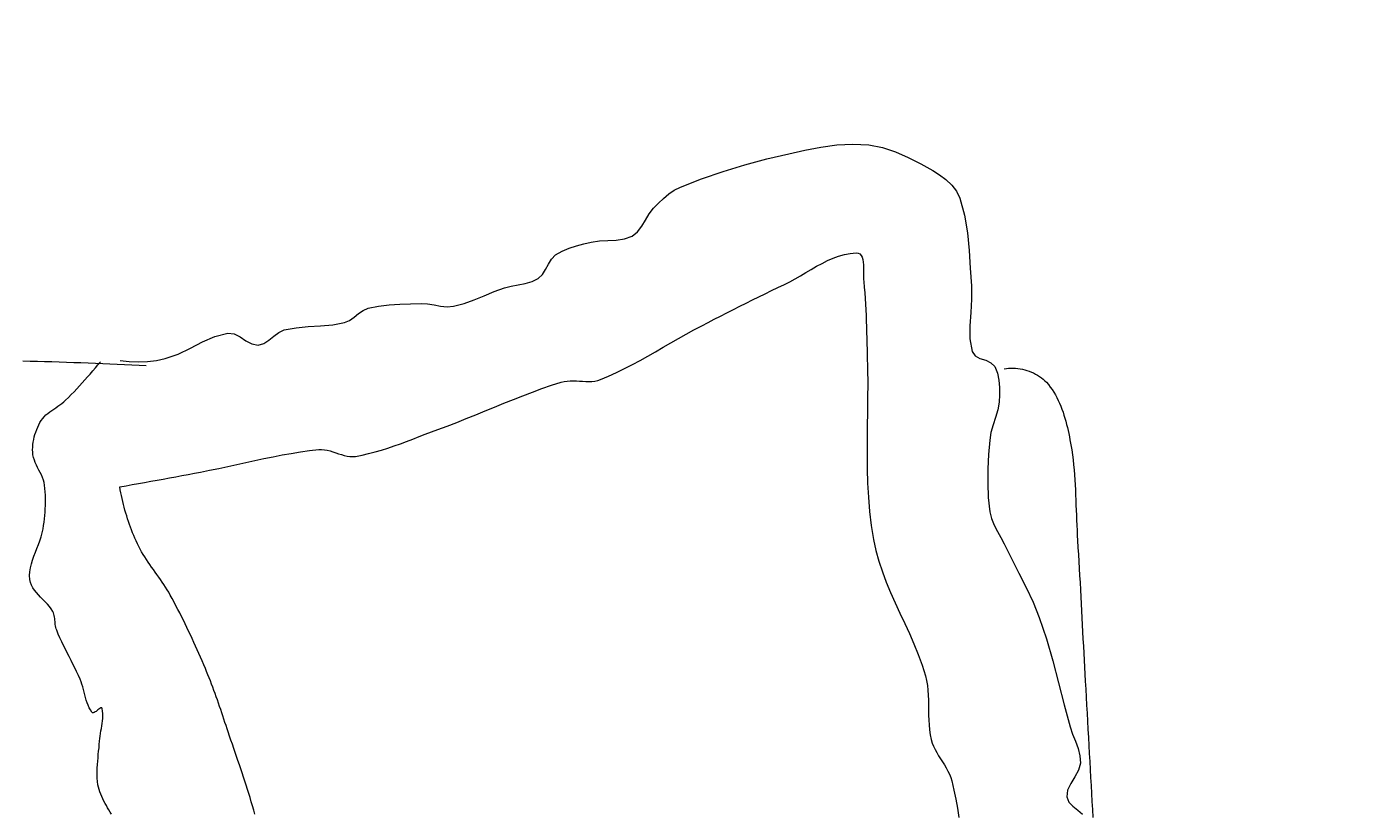
# Model space of a CAD drawing. Units: inches. Extents: x 1441 to 2460, y 1648 to 2683.
# Tile 8 of 35: x 1852 to 1880, y 1917 to 1933. Entities that reach past the tile are written whole.
import ezdxf

# ---------------------------------------------------------------- set-up
doc = ezdxf.new("R2010")
doc.units = ezdxf.units.IN
doc.layers.add('A-ANNO-DIMS', color=2, linetype='Continuous', lineweight=18)
doc.layers.add('A-FURN', color=8, linetype='Continuous', lineweight=15)
doc.styles.get("Standard").update_dxf_attribs({"font": 'arial.ttf'})
doc.dimstyles.get("Standard").update_dxf_attribs({"dimtxt": 0.18, "dimasz": 0.18, "dimexe": 0.18, "dimexo": 0.0625, "dimgap": 0.09, "dimtad": 0, "dimtih": 1, "dimtoh": 1, "dimdec": 4, "dimzin": 0, "dimdsep": 46, "dimtxsty": 'Standard', "dimcen": 0.09, "dimadec": 0, "dimazin": 0, "dimtfac": 1, "dimtdec": 4, "dimtofl": 0, "dimtmove": 0, "dimatfit": 3, "dimfxl": 1, "dimtolj": 1, "dimtzin": 0, "dimarcsym": 0})

# ---------------------------------------------------------------- blocks, each defined once
blk = doc.blocks.new('BED-DOUBLE-PLAN')
for p, q in [((13.358, 86.279), (13.525, 86.288)), ((13.525, 86.288), (13.692, 86.298)), ((13.692, 86.298), (13.859, 86.307)), ((13.859, 86.307), (14.025, 86.316)), ((14.025, 86.316), (14.192, 86.326)), ((14.192, 86.326), (14.359, 86.335)), ((14.359, 86.335), (14.526, 86.344)), ((14.526, 86.344), (14.693, 86.354)), ((14.693, 86.354), (14.859, 86.363)), ((14.859, 86.363), (15.026, 86.373)), ((15.026, 86.373), (15.193, 86.382)), ((15.193, 86.382), (15.36, 86.392)), ((8.125, 86), (8.23, 86.008)), ((8.23, 86.008), (8.334, 86.016)), ((8.334, 86.016), (8.439, 86.022)), ((8.439, 86.022), (8.544, 86.028)), ((8.544, 86.028), (8.649, 86.032)), ((8.649, 86.032), (8.755, 86.037)), ((8.755, 86.037), (8.86, 86.04)), ((8.86, 86.04), (8.965, 86.044)), ((8.965, 86.044), (9.07, 86.048)), ((9.07, 86.048), (9.175, 86.052)), ((9.175, 86.052), (9.281, 86.056)), ((9.281, 86.056), (9.386, 86.061)), ((9.386, 86.061), (9.491, 86.066)), ((9.491, 86.066), (9.595, 86.072)), ((9.595, 86.072), (9.742, 86.081)), ((9.742, 86.081), (9.888, 86.09)), ((9.888, 86.09), (10.035, 86.099)), ((10.035, 86.099), (10.181, 86.107)), ((10.181, 86.107), (10.327, 86.116)), ((10.327, 86.116), (10.474, 86.124)), ((10.474, 86.124), (10.62, 86.132)), ((10.62, 86.132), (10.767, 86.14)), ((10.767, 86.14), (10.913, 86.147)), ((10.913, 86.147), (11.059, 86.155)), ((11.059, 86.155), (11.206, 86.163)), ((11.206, 86.163), (11.352, 86.17)), ((11.352, 86.17), (11.499, 86.178)), ((11.499, 86.178), (11.645, 86.185)), ((11.645, 86.185), (11.792, 86.193)), ((11.792, 86.193), (11.938, 86.201)), ((11.938, 86.201), (12.085, 86.209)), ((12.085, 86.209), (12.231, 86.216)), ((12.231, 86.216), (12.377, 86.224)), ((12.377, 86.224), (12.524, 86.232)), ((12.524, 86.232), (12.691, 86.242)), ((12.691, 86.242), (12.858, 86.251)), ((12.858, 86.251), (13.024, 86.26)), ((13.024, 86.26), (13.191, 86.27)), ((13.191, 86.27), (13.358, 86.279)), ((13.624, 85.969), (13.774, 86.028)), ((13.774, 86.028), (13.925, 86.082)), ((13.925, 86.082), (14.077, 86.121)), ((14.077, 86.121), (14.232, 86.132)), ((14.232, 86.132), (14.378, 86.095)), ((14.378, 86.095), (14.515, 86.019)), ((14.515, 86.019), (14.65, 85.933)), ((15.126, 85.971), (15.205, 86.075)), ((15.205, 86.075), (15.287, 86.175)), ((6.802, 85.724), (6.864, 85.748)), ((6.864, 85.748), (6.926, 85.77)), ((6.926, 85.77), (6.989, 85.79)), ((6.989, 85.79), (7.053, 85.809)), ((7.053, 85.809), (7.117, 85.827)), ((7.117, 85.827), (7.181, 85.844)), ((7.181, 85.844), (7.246, 85.86)), ((7.246, 85.86), (7.31, 85.874)), ((7.31, 85.874), (7.374, 85.888)), ((7.374, 85.888), (7.438, 85.902)), ((7.438, 85.902), (7.502, 85.915)), ((7.502, 85.915), (7.605, 85.934)), ((7.605, 85.934), (7.709, 85.951)), ((7.709, 85.951), (7.812, 85.966)), ((7.812, 85.966), (7.916, 85.979)), ((7.916, 85.979), (8.021, 85.99)), ((8.021, 85.99), (8.125, 86)), ((12.558, 85.676), (13.016, 85.794)), ((13.016, 85.794), (13.473, 85.918)), ((13.473, 85.918), (13.624, 85.969)), ((14.65, 85.933), (14.788, 85.865)), ((14.788, 85.865), (14.932, 85.847)), ((14.932, 85.847), (15.039, 85.888)), ((15.039, 85.888), (15.126, 85.971)), ((6.306, 85.423), (6.354, 85.466)), ((6.354, 85.466), (6.405, 85.506)), ((6.405, 85.506), (6.457, 85.544)), ((6.457, 85.544), (6.511, 85.579)), ((6.511, 85.579), (6.567, 85.612)), ((6.567, 85.612), (6.624, 85.643)), ((6.624, 85.643), (6.682, 85.672)), ((6.682, 85.672), (6.742, 85.699)), ((6.742, 85.699), (6.802, 85.724)), ((11.645, 85.425), (12.1, 85.556)), ((12.1, 85.556), (12.558, 85.676)), ((6.112, 85.155), (6.134, 85.199)), ((6.134, 85.199), (6.158, 85.24)), ((6.158, 85.24), (6.184, 85.281)), ((6.184, 85.281), (6.212, 85.319)), ((6.212, 85.319), (6.241, 85.356)), ((6.241, 85.356), (6.273, 85.391)), ((6.273, 85.391), (6.306, 85.423)), ((10.883, 85.149), (11.197, 85.276)), ((11.197, 85.276), (11.645, 85.425)), ((6.023, 84.877), (6.032, 84.924)), ((6.032, 84.924), (6.044, 84.972)), ((6.044, 84.972), (6.057, 85.019)), ((6.057, 85.019), (6.073, 85.065)), ((6.073, 85.065), (6.092, 85.111)), ((6.092, 85.111), (6.112, 85.155)), ((10.274, 84.851), (10.576, 85.005)), ((10.576, 85.005), (10.883, 85.149)), ((6.009, 84.732), (6.011, 84.78)), ((6.009, 84.685), (6.009, 84.732)), ((6.012, 84.638), (6.009, 84.685)), ((6.011, 84.78), (6.015, 84.828)), ((6.017, 84.591), (6.012, 84.638)), ((6.015, 84.828), (6.023, 84.877)), ((9.668, 84.546), (9.972, 84.695)), ((9.972, 84.695), (10.274, 84.851)), ((5.898, 84.271), (5.976, 84.349)), ((5.976, 84.349), (6.115, 84.405)), ((6.025, 84.546), (6.017, 84.591)), ((6.115, 84.405), (6.262, 84.436)), ((6.262, 84.436), (6.415, 84.448)), ((6.415, 84.448), (6.569, 84.447)), ((6.569, 84.447), (6.721, 84.438)), ((6.721, 84.438), (6.88, 84.413)), ((6.88, 84.413), (7.036, 84.368)), ((7.036, 84.368), (7.192, 84.317)), ((9.141, 84.279), (9.276, 84.335)), ((9.276, 84.335), (9.407, 84.405)), ((9.407, 84.405), (9.537, 84.478)), ((9.537, 84.478), (9.668, 84.546)), ((5.807, 84.042), (5.848, 84.161)), ((5.848, 84.161), (5.898, 84.271)), ((7.192, 84.317), (7.348, 84.271)), ((7.348, 84.271), (7.507, 84.244)), ((7.507, 84.244), (7.806, 84.221)), ((7.806, 84.221), (8.105, 84.206)), ((8.105, 84.206), (8.405, 84.203)), ((8.405, 84.203), (8.703, 84.214)), ((8.703, 84.214), (9, 84.245)), ((9, 84.245), (9.141, 84.279)), ((2.83, 83.719), (3.193, 83.779)), ((3.193, 83.779), (3.561, 83.814)), ((3.561, 83.814), (3.931, 83.839)), ((3.931, 83.839), (4.3, 83.864)), ((4.3, 83.864), (4.575, 83.867)), ((4.575, 83.867), (4.852, 83.849)), ((4.852, 83.849), (5.128, 83.83)), ((5.128, 83.83), (5.401, 83.833)), ((5.401, 83.833), (5.668, 83.879)), ((5.668, 83.879), (5.753, 83.94)), ((5.753, 83.94), (5.807, 84.042)), ((2.203, 83.455), (2.331, 83.555)), ((2.331, 83.555), (2.475, 83.624)), ((2.475, 83.624), (2.83, 83.719)), ((14.6, 83.457), (14.788, 83.501)), ((14.788, 83.501), (14.977, 83.539)), ((14.977, 83.539), (15.168, 83.572)), ((15.168, 83.572), (15.359, 83.6)), ((1.99, 83.199), (2.089, 83.333)), ((2.089, 83.333), (2.203, 83.455)), ((14.074, 83.182), (14.138, 83.222)), ((14.138, 83.222), (14.201, 83.262)), ((14.201, 83.262), (14.265, 83.302)), ((14.265, 83.302), (14.329, 83.341)), ((14.329, 83.341), (14.394, 83.376)), ((14.394, 83.376), (14.461, 83.408)), ((14.461, 83.408), (14.529, 83.436)), ((14.529, 83.436), (14.6, 83.457)), ((1.759, 82.808), (1.902, 83.059)), ((1.902, 83.059), (1.99, 83.199)), ((12.409, 82.906), (12.509, 82.931)), ((12.509, 82.931), (12.61, 82.948)), ((12.61, 82.948), (12.711, 82.96)), ((12.711, 82.96), (12.814, 82.967)), ((12.814, 82.967), (12.917, 82.971)), ((12.917, 82.971), (13.021, 82.972)), ((13.021, 82.972), (13.125, 82.973)), ((13.125, 82.973), (13.229, 82.974)), ((13.229, 82.974), (13.332, 82.976)), ((13.332, 82.976), (13.435, 82.982)), ((13.435, 82.982), (13.538, 82.991)), ((13.538, 82.991), (13.639, 83.006)), ((13.639, 83.006), (13.739, 83.027)), ((13.739, 83.027), (13.81, 83.049)), ((13.81, 83.049), (13.878, 83.076)), ((13.878, 83.076), (13.945, 83.108)), ((13.945, 83.108), (14.01, 83.144)), ((14.01, 83.144), (14.074, 83.182)), ((1.626, 82.55), (1.759, 82.808)), ((11.535, 82.573), (11.75, 82.667)), ((11.75, 82.667), (11.967, 82.755)), ((11.967, 82.755), (12.187, 82.836)), ((12.187, 82.836), (12.409, 82.906)), ((1.51, 82.285), (1.626, 82.55)), ((10.894, 82.279), (11.108, 82.377)), ((11.108, 82.377), (11.321, 82.476)), ((11.321, 82.476), (11.535, 82.573)), ((1.42, 82.012), (1.51, 82.285)), ((10.246, 82.01), (10.464, 82.093)), ((10.464, 82.093), (10.679, 82.183)), ((10.679, 82.183), (10.894, 82.279)), ((1.366, 81.731), (1.42, 82.012)), ((9.283, 81.778), (9.574, 81.824)), ((9.574, 81.824), (9.802, 81.873)), ((9.802, 81.873), (10.026, 81.936)), ((10.026, 81.936), (10.246, 82.01)), ((1.348, 81.397), (1.366, 81.731)), ((3.617, 81.509), (3.635, 81.543)), ((3.635, 81.543), (3.665, 81.569)), ((3.665, 81.569), (3.704, 81.588)), ((3.704, 81.588), (3.751, 81.602)), ((3.751, 81.602), (3.804, 81.61)), ((3.804, 81.61), (3.862, 81.615)), ((3.862, 81.615), (3.922, 81.618)), ((3.922, 81.618), (3.984, 81.618)), ((3.984, 81.618), (4.046, 81.618)), ((4.046, 81.618), (4.106, 81.618)), ((4.106, 81.618), (4.162, 81.619)), ((4.162, 81.619), (4.212, 81.623)), ((4.212, 81.623), (4.329, 81.634)), ((4.329, 81.634), (4.446, 81.644)), ((4.446, 81.644), (4.564, 81.652)), ((4.564, 81.652), (4.681, 81.659)), ((4.681, 81.659), (4.798, 81.665)), ((4.798, 81.665), (4.916, 81.67)), ((4.916, 81.67), (5.033, 81.674)), ((5.033, 81.674), (5.151, 81.678)), ((5.151, 81.678), (5.269, 81.681)), ((5.269, 81.681), (5.386, 81.684)), ((5.386, 81.684), (5.504, 81.688)), ((5.504, 81.688), (5.621, 81.691)), ((5.621, 81.691), (5.739, 81.695)), ((5.739, 81.695), (6.034, 81.703)), ((6.034, 81.703), (6.33, 81.706)), ((6.33, 81.706), (6.626, 81.704)), ((6.626, 81.704), (6.923, 81.701)), ((6.923, 81.701), (7.219, 81.696)), ((7.219, 81.696), (7.516, 81.693)), ((7.516, 81.693), (7.812, 81.692)), ((7.812, 81.692), (8.108, 81.695)), ((8.108, 81.695), (8.403, 81.703)), ((8.403, 81.703), (8.697, 81.719)), ((8.697, 81.719), (8.991, 81.743)), ((8.991, 81.743), (9.283, 81.778)), ((1.367, 81.062), (1.348, 81.397)), ((3.612, 81.466), (3.617, 81.509)), ((3.623, 81.342), (3.612, 81.466)), ((3.646, 81.22), (3.623, 81.342)), ((1.413, 80.727), (1.367, 81.062)), ((3.68, 81.101), (3.646, 81.22)), ((3.723, 80.984), (3.68, 81.101)), ((3.774, 80.869), (3.723, 80.984)), ((1.477, 80.394), (1.413, 80.727)), ((3.831, 80.755), (3.774, 80.869)), ((3.892, 80.643), (3.831, 80.755)), ((3.957, 80.531), (3.892, 80.643)), ((4.023, 80.419), (3.957, 80.531)), ((4.088, 80.308), (4.023, 80.419)), ((1.549, 80.065), (1.477, 80.394)), ((4.153, 80.196), (4.088, 80.308)), ((4.214, 80.084), (4.153, 80.196)), ((1.659, 79.605), (1.549, 80.065)), ((4.27, 79.971), (4.214, 80.084)), ((4.334, 79.837), (4.27, 79.971)), ((1.783, 79.148), (1.659, 79.605)), ((4.398, 79.704), (4.334, 79.837)), ((4.462, 79.571), (4.398, 79.704)), ((4.527, 79.438), (4.462, 79.571)), ((4.593, 79.305), (4.527, 79.438)), ((4.659, 79.173), (4.593, 79.305)), ((1.921, 78.696), (1.783, 79.148)), ((4.725, 79.041), (4.659, 79.173)), ((4.792, 78.909), (4.725, 79.041)), ((4.859, 78.777), (4.792, 78.909)), ((4.927, 78.645), (4.859, 78.777)), ((2.075, 78.248), (1.921, 78.696)), ((4.994, 78.513), (4.927, 78.645)), ((5.062, 78.382), (4.994, 78.513)), ((2.244, 77.807), (2.075, 78.248)), ((5.13, 78.25), (5.062, 78.382)), ((5.215, 78.088), (5.13, 78.25)), ((5.304, 77.927), (5.215, 78.088)), ((5.394, 77.767), (5.304, 77.927)), ((2.307, 77.68), (2.244, 77.807)), ((2.388, 77.564), (2.307, 77.68)), ((5.485, 77.608), (5.394, 77.767)), ((5.577, 77.449), (5.485, 77.608)), ((2.481, 77.454), (2.388, 77.564)), ((2.582, 77.35), (2.481, 77.454)), ((2.684, 77.249), (2.582, 77.35)), ((5.669, 77.289), (5.577, 77.449)), ((2.8, 77.157), (2.684, 77.249)), ((2.929, 77.079), (2.8, 77.157)), ((3.059, 77.002), (2.929, 77.079)), ((5.759, 77.13), (5.669, 77.289)), ((5.849, 76.969), (5.759, 77.13)), ((3.175, 76.914), (3.059, 77.002)), ((3.263, 76.801), (3.175, 76.914)), ((3.323, 76.643), (3.263, 76.801)), ((5.936, 76.808), (5.849, 76.969)), ((6.02, 76.645), (5.936, 76.808)), ((3.348, 76.473), (3.323, 76.643)), ((6.1, 76.48), (6.02, 76.645)), ((6.176, 76.314), (6.1, 76.48)), ((3.356, 76.298), (3.348, 76.473)), ((3.364, 76.122), (3.356, 76.298)), ((6.247, 76.145), (6.176, 76.314)), ((3.391, 75.951), (3.364, 76.122)), ((3.428, 75.797), (3.391, 75.951)), ((6.267, 76.086), (6.247, 76.145)), ((6.28, 76.025), (6.267, 76.086)), ((6.286, 75.963), (6.28, 76.025)), ((6.289, 75.9), (6.286, 75.963)), ((3.469, 75.643), (3.428, 75.797)), ((3.518, 75.492), (3.469, 75.643)), ((6.275, 75.579), (6.277, 75.643)), ((6.277, 75.643), (6.281, 75.708)), ((6.281, 75.708), (6.285, 75.772)), ((6.285, 75.772), (6.288, 75.836)), ((6.288, 75.836), (6.289, 75.9)), ((3.579, 75.347), (3.518, 75.492)), ((6.275, 75.515), (6.275, 75.579)), ((6.279, 75.452), (6.275, 75.515)), ((6.288, 75.39), (6.279, 75.452)), ((6.303, 75.329), (6.288, 75.39)), ((3.657, 75.211), (3.579, 75.347)), ((3.742, 75.126), (3.657, 75.211)), ((3.848, 75.061), (3.742, 75.126)), ((6.367, 75.127), (6.303, 75.329)), ((6.436, 74.927), (6.367, 75.127)), ((3.96, 75.003), (3.848, 75.061)), ((4.064, 74.937), (3.96, 75.003)), ((4.146, 74.85), (4.064, 74.937)), ((4.21, 74.72), (4.146, 74.85)), ((6.508, 74.728), (6.436, 74.927)), ((4.25, 74.579), (4.21, 74.72)), ((4.278, 74.433), (4.25, 74.579)), ((6.584, 74.53), (6.508, 74.728)), ((6.661, 74.333), (6.584, 74.53)), ((4.304, 74.287), (4.278, 74.433)), ((4.341, 74.144), (4.304, 74.287)), ((6.74, 74.136), (6.661, 74.333)), ((4.419, 73.932), (4.341, 74.144)), ((6.821, 73.94), (6.74, 74.136)), ((4.506, 73.724), (4.419, 73.932)), ((4.592, 73.515), (4.506, 73.724)), ((6.901, 73.744), (6.821, 73.94)), ((6.982, 73.548), (6.901, 73.744)), ((4.667, 73.304), (4.592, 73.515)), ((7.062, 73.352), (6.982, 73.548)), ((4.722, 73.087), (4.667, 73.304)), ((7.14, 73.155), (7.062, 73.352)), ((7.216, 72.957), (7.14, 73.155)), ((4.72, 72.818), (4.732, 72.953)), ((4.732, 72.953), (4.722, 73.087)), ((7.289, 72.758), (7.216, 72.957)), ((4.675, 72.546), (4.697, 72.682)), ((4.697, 72.682), (4.72, 72.818)), ((7.337, 72.628), (7.289, 72.758)), ((7.386, 72.498), (7.337, 72.628)), ((4.668, 72.41), (4.675, 72.546)), ((4.673, 72.189), (4.668, 72.41)), ((7.436, 72.369), (7.386, 72.498)), ((7.486, 72.239), (7.436, 72.369)), ((4.68, 71.967), (4.673, 72.189)), ((7.535, 72.109), (7.486, 72.239)), ((7.583, 71.979), (7.535, 72.109)), ((4.695, 71.746), (4.68, 71.967)), ((4.722, 71.527), (4.695, 71.746)), ((7.63, 71.848), (7.583, 71.979)), ((7.675, 71.717), (7.63, 71.848)), ((4.765, 71.311), (4.722, 71.527)), ((7.717, 71.585), (7.675, 71.717)), ((7.755, 71.452), (7.717, 71.585)), ((7.79, 71.318), (7.755, 71.452)), ((4.809, 71.206), (4.765, 71.311)), ((4.876, 71.111), (4.809, 71.206)), ((7.821, 71.184), (7.79, 71.318)), ((7.846, 71.048), (7.821, 71.184)), ((4.95, 71.019), (4.876, 71.111)), ((5.017, 70.924), (4.95, 71.019)), ((5.062, 70.82), (5.017, 70.924)), ((7.842, 70.871), (7.85, 70.93)), ((7.852, 70.989), (7.846, 71.048)), ((7.85, 70.93), (7.852, 70.989)), ((5.108, 70.571), (5.062, 70.82)), ((7.752, 70.577), (7.772, 70.636)), ((7.772, 70.636), (7.792, 70.694)), ((7.792, 70.694), (7.811, 70.753)), ((7.811, 70.753), (7.828, 70.812)), ((7.828, 70.812), (7.842, 70.871)), ((5.131, 70.318), (5.108, 70.571)), ((5.147, 70.064), (5.131, 70.318)), ((7.703, 70.34), (7.708, 70.399)), ((7.705, 70.28), (7.703, 70.34)), ((7.708, 70.399), (7.719, 70.459)), ((7.719, 70.459), (7.734, 70.518)), ((7.734, 70.518), (7.752, 70.577)), ((5.17, 69.811), (5.147, 70.064)), ((7.727, 70.089), (7.705, 70.28)), ((7.754, 69.899), (7.727, 70.089)), ((5.217, 69.562), (5.17, 69.811)), ((7.784, 69.709), (7.754, 69.899)), ((5.269, 69.448), (5.217, 69.562)), ((7.818, 69.519), (7.784, 69.709)), ((7.855, 69.33), (7.818, 69.519)), ((5.347, 69.344), (5.269, 69.448)), ((5.431, 69.242), (5.347, 69.344)), ((5.5, 69.136), (5.431, 69.242)), ((7.893, 69.141), (7.855, 69.33)), ((5.532, 69.019), (5.5, 69.136)), ((5.508, 68.888), (5.532, 69.019)), ((7.934, 68.953), (7.893, 69.141)), ((7.975, 68.764), (7.934, 68.953)), ((15.204, 68.929), (15.118, 68.903)), ((15.29, 68.954), (15.204, 68.929)), ((5.296, 68.52), (5.359, 68.643)), ((5.359, 68.643), (5.44, 68.765)), ((5.44, 68.765), (5.508, 68.888)), ((8.017, 68.576), (7.975, 68.764)), ((14.347, 68.657), (14.262, 68.629)), ((14.432, 68.686), (14.347, 68.657)), ((14.518, 68.714), (14.432, 68.686)), ((14.603, 68.742), (14.518, 68.714)), ((14.689, 68.769), (14.603, 68.742)), ((14.774, 68.797), (14.689, 68.769)), ((14.86, 68.824), (14.774, 68.797)), ((14.946, 68.851), (14.86, 68.824)), ((15.032, 68.877), (14.946, 68.851)), ((15.118, 68.903), (15.032, 68.877)), ((5.281, 68.391), (5.296, 68.52)), ((5.35, 68.121), (5.281, 68.391)), ((8.058, 68.388), (8.017, 68.576)), ((8.098, 68.199), (8.058, 68.388)), ((13.514, 68.375), (13.447, 68.352)), ((13.58, 68.397), (13.514, 68.375)), ((13.665, 68.426), (13.58, 68.397)), ((13.75, 68.455), (13.665, 68.426)), ((13.836, 68.484), (13.75, 68.455)), ((13.921, 68.513), (13.836, 68.484)), ((14.006, 68.542), (13.921, 68.513)), ((14.091, 68.571), (14.006, 68.542)), ((14.176, 68.6), (14.091, 68.571)), ((14.262, 68.629), (14.176, 68.6)), ((5.463, 67.863), (5.35, 68.121)), ((8.137, 68.01), (8.098, 68.199)), ((12.651, 68.076), (12.585, 68.051)), ((12.717, 68.1), (12.651, 68.076)), ((12.783, 68.124), (12.717, 68.1)), ((12.849, 68.148), (12.783, 68.124)), ((12.915, 68.171), (12.849, 68.148)), ((12.981, 68.194), (12.915, 68.171)), ((13.048, 68.217), (12.981, 68.194)), ((13.114, 68.24), (13.048, 68.217)), ((13.181, 68.262), (13.114, 68.24)), ((13.247, 68.285), (13.181, 68.262)), ((13.314, 68.307), (13.247, 68.285)), ((13.381, 68.33), (13.314, 68.307)), ((13.447, 68.352), (13.381, 68.33)), ((5.593, 67.609), (5.463, 67.863)), ((8.174, 67.821), (8.137, 68.01)), ((8.198, 67.692), (8.174, 67.821)), ((12.025, 67.82), (11.948, 67.786)), ((12.103, 67.854), (12.025, 67.82)), ((12.181, 67.888), (12.103, 67.854)), ((12.259, 67.921), (12.181, 67.888)), ((12.324, 67.948), (12.259, 67.921)), ((12.389, 67.974), (12.324, 67.948)), ((12.454, 68.001), (12.389, 67.974)), ((12.519, 68.026), (12.454, 68.001)), ((12.585, 68.051), (12.519, 68.026)), ((5.717, 67.354), (5.593, 67.609)), ((8.222, 67.563), (8.198, 67.692)), ((8.246, 67.434), (8.222, 67.563)), ((11.409, 67.538), (11.333, 67.501)), ((11.486, 67.574), (11.409, 67.538)), ((11.562, 67.611), (11.486, 67.574)), ((11.639, 67.646), (11.562, 67.611)), ((11.716, 67.682), (11.639, 67.646)), ((11.793, 67.717), (11.716, 67.682)), ((11.87, 67.752), (11.793, 67.717)), ((11.948, 67.786), (11.87, 67.752)), ((5.81, 67.088), (5.717, 67.354)), ((8.27, 67.304), (8.246, 67.434)), ((8.294, 67.175), (8.27, 67.304)), ((10.88, 67.271), (10.805, 67.231)), ((10.955, 67.31), (10.88, 67.271)), ((11.03, 67.349), (10.955, 67.31)), ((11.105, 67.388), (11.03, 67.349)), ((11.181, 67.426), (11.105, 67.388)), ((11.257, 67.464), (11.181, 67.426)), ((11.333, 67.501), (11.257, 67.464)), ((5.849, 66.904), (5.81, 67.088)), ((8.318, 67.046), (8.294, 67.175)), ((8.341, 66.917), (8.318, 67.046)), ((10.409, 66.988), (10.357, 66.951)), ((10.461, 67.024), (10.409, 66.988)), ((10.514, 67.059), (10.461, 67.024)), ((10.567, 67.094), (10.514, 67.059)), ((10.621, 67.127), (10.567, 67.094)), ((10.675, 67.159), (10.621, 67.127)), ((10.731, 67.191), (10.675, 67.159)), ((10.805, 67.231), (10.731, 67.191)), ((5.873, 66.715), (5.849, 66.904)), ((5.881, 66.525), (5.873, 66.715)), ((5.946, 66.541), (5.953, 66.692)), ((8.365, 66.787), (8.341, 66.917)), ((8.388, 66.658), (8.365, 66.787)), ((9.992, 66.695), (9.939, 66.661)), ((10.045, 66.731), (9.992, 66.695)), ((10.097, 66.767), (10.045, 66.731)), ((10.149, 66.803), (10.097, 66.767)), ((10.201, 66.84), (10.149, 66.803)), ((10.253, 66.877), (10.201, 66.84)), ((10.305, 66.914), (10.253, 66.877)), ((10.357, 66.951), (10.305, 66.914)), ((5.874, 66.335), (5.881, 66.525)), ((5.939, 66.39), (5.946, 66.541)), ((8.412, 66.529), (8.388, 66.658)), ((8.435, 66.399), (8.412, 66.529)), ((8.458, 66.27), (8.435, 66.399)), ((9.436, 66.408), (9.378, 66.386)), ((9.493, 66.432), (9.436, 66.408)), ((9.55, 66.456), (9.493, 66.432)), ((9.607, 66.481), (9.55, 66.456)), ((9.663, 66.507), (9.607, 66.481)), ((9.72, 66.535), (9.663, 66.507)), ((9.776, 66.564), (9.72, 66.535)), ((9.831, 66.595), (9.776, 66.564)), ((9.886, 66.627), (9.831, 66.595)), ((9.939, 66.661), (9.886, 66.627)), ((5.851, 66.148), (5.874, 66.335)), ((5.926, 66.088), (5.932, 66.239)), ((5.932, 66.239), (5.939, 66.39)), ((8.481, 66.141), (8.458, 66.27)), ((8.542, 66.151), (8.481, 66.141)), ((8.603, 66.163), (8.542, 66.151)), ((8.664, 66.175), (8.603, 66.163)), ((8.725, 66.188), (8.664, 66.175)), ((8.785, 66.202), (8.725, 66.188)), ((8.845, 66.216), (8.785, 66.202)), ((8.905, 66.232), (8.845, 66.216)), ((8.965, 66.248), (8.905, 66.232)), ((9.025, 66.266), (8.965, 66.248)), ((9.085, 66.284), (9.025, 66.266)), ((9.144, 66.303), (9.085, 66.284)), ((9.203, 66.322), (9.144, 66.303)), ((9.262, 66.342), (9.203, 66.322)), ((9.32, 66.364), (9.262, 66.342)), ((9.378, 66.386), (9.32, 66.364)), ((5.913, 65.785), (5.92, 65.936)), ((5.92, 65.936), (5.926, 66.088)), ((15.066, 65.835), (15.019, 65.81)), ((15.112, 65.861), (15.066, 65.835)), ((15.157, 65.887), (15.112, 65.861)), ((15.202, 65.914), (15.157, 65.887)), ((15.247, 65.942), (15.202, 65.914)), ((15.292, 65.969), (15.247, 65.942)), ((5.943, 65.687), (5.879, 65.74)), ((5.902, 65.483), (5.908, 65.634)), ((5.908, 65.634), (5.913, 65.785)), ((6.006, 65.633), (5.943, 65.687)), ((6.07, 65.579), (6.006, 65.633)), ((6.133, 65.525), (6.07, 65.579)), ((13.081, 65.766), (13.078, 65.756)), ((13.078, 65.756), (13.081, 65.742)), ((13.093, 65.773), (13.081, 65.766)), ((13.081, 65.742), (13.09, 65.726)), ((13.09, 65.726), (13.103, 65.707)), ((13.144, 65.784), (13.093, 65.773)), ((13.103, 65.707), (13.118, 65.687)), ((13.118, 65.687), (13.135, 65.667)), ((13.169, 65.562), (13.123, 65.53)), ((13.135, 65.667), (13.151, 65.646)), ((13.195, 65.789), (13.144, 65.784)), ((13.151, 65.646), (13.164, 65.626)), ((13.164, 65.626), (13.175, 65.606)), ((13.179, 65.574), (13.169, 65.562)), ((13.175, 65.606), (13.18, 65.589)), ((13.18, 65.589), (13.179, 65.574)), ((13.247, 65.791), (13.195, 65.789)), ((13.298, 65.788), (13.247, 65.791)), ((13.35, 65.783), (13.298, 65.788)), ((13.403, 65.776), (13.35, 65.783)), ((13.455, 65.767), (13.403, 65.776)), ((13.508, 65.757), (13.455, 65.767)), ((13.56, 65.747), (13.508, 65.757)), ((13.613, 65.738), (13.56, 65.747)), ((13.665, 65.729), (13.613, 65.738)), ((13.718, 65.723), (13.665, 65.729)), ((13.77, 65.718), (13.718, 65.723)), ((13.84, 65.714), (13.77, 65.718)), ((13.91, 65.708), (13.84, 65.714)), ((13.98, 65.701), (13.91, 65.708)), ((14.05, 65.694), (13.98, 65.701)), ((14.12, 65.688), (14.05, 65.694)), ((14.19, 65.681), (14.12, 65.688)), ((14.26, 65.676), (14.19, 65.681)), ((14.33, 65.672), (14.26, 65.676)), ((14.399, 65.669), (14.33, 65.672)), ((14.469, 65.669), (14.399, 65.669)), ((14.539, 65.672), (14.469, 65.669)), ((14.608, 65.678), (14.539, 65.672)), ((14.677, 65.687), (14.608, 65.678)), ((14.728, 65.697), (14.677, 65.687)), ((14.778, 65.71), (14.728, 65.697)), ((14.828, 65.726), (14.778, 65.71)), ((14.876, 65.744), (14.828, 65.726)), ((14.924, 65.764), (14.876, 65.744)), ((14.972, 65.786), (14.924, 65.764)), ((15.019, 65.81), (14.972, 65.786)), ((5.891, 65.181), (5.896, 65.332)), ((5.896, 65.332), (5.902, 65.483)), ((6.195, 65.47), (6.133, 65.525)), ((6.257, 65.414), (6.195, 65.47)), ((6.319, 65.358), (6.257, 65.414)), ((6.38, 65.302), (6.319, 65.358)), ((6.44, 65.245), (6.38, 65.302)), ((12.403, 65.279), (12.324, 65.242)), ((12.482, 65.314), (12.403, 65.279)), ((12.535, 65.335), (12.482, 65.314)), ((12.588, 65.353), (12.535, 65.335)), ((12.643, 65.369), (12.588, 65.353)), ((12.698, 65.384), (12.643, 65.369)), ((12.754, 65.398), (12.698, 65.384)), ((12.809, 65.412), (12.754, 65.398)), ((12.864, 65.426), (12.809, 65.412)), ((12.919, 65.442), (12.864, 65.426)), ((12.972, 65.46), (12.919, 65.442)), ((13.024, 65.48), (12.972, 65.46)), ((13.075, 65.503), (13.024, 65.48)), ((13.123, 65.53), (13.075, 65.503)), ((5.881, 64.878), (5.886, 65.029)), ((5.886, 65.029), (5.891, 65.181)), ((6.501, 65.188), (6.44, 65.245)), ((6.56, 65.13), (6.501, 65.188)), ((6.619, 65.071), (6.56, 65.13)), ((6.678, 65.013), (6.619, 65.071)), ((6.713, 64.975), (6.678, 65.013)), ((11.858, 65.008), (11.78, 64.97)), ((11.935, 65.048), (11.858, 65.008)), ((12.013, 65.087), (11.935, 65.048)), ((12.09, 65.127), (12.013, 65.087)), ((12.168, 65.166), (12.09, 65.127)), ((12.246, 65.204), (12.168, 65.166)), ((12.324, 65.242), (12.246, 65.204)), ((5.872, 64.576), (5.876, 64.727)), ((5.876, 64.727), (5.881, 64.878)), ((6.745, 64.936), (6.713, 64.975)), ((6.776, 64.895), (6.745, 64.936)), ((6.805, 64.853), (6.776, 64.895)), ((6.834, 64.81), (6.805, 64.853)), ((6.863, 64.767), (6.834, 64.81)), ((6.892, 64.724), (6.863, 64.767)), ((6.922, 64.683), (6.892, 64.724)), ((11.02, 64.714), (10.969, 64.676)), ((11.074, 64.746), (11.02, 64.714)), ((11.102, 64.759), (11.074, 64.746)), ((11.13, 64.769), (11.102, 64.759)), ((11.16, 64.777), (11.13, 64.769)), ((11.19, 64.782), (11.16, 64.777)), ((11.22, 64.787), (11.19, 64.782)), ((11.251, 64.79), (11.22, 64.787)), ((11.282, 64.793), (11.251, 64.79)), ((11.313, 64.796), (11.282, 64.793)), ((11.344, 64.799), (11.313, 64.796)), ((11.375, 64.803), (11.344, 64.799)), ((11.405, 64.809), (11.375, 64.803)), ((11.435, 64.817), (11.405, 64.809)), ((11.463, 64.827), (11.435, 64.817)), ((11.544, 64.86), (11.463, 64.827)), ((11.623, 64.896), (11.544, 64.86)), ((11.702, 64.932), (11.623, 64.896)), ((11.78, 64.97), (11.702, 64.932)), ((5.868, 64.425), (5.872, 64.576)), ((6.953, 64.643), (6.922, 64.683)), ((6.985, 64.605), (6.953, 64.643)), ((7.021, 64.569), (6.985, 64.605)), ((7.058, 64.536), (7.021, 64.569)), ((7.099, 64.507), (7.058, 64.536)), ((7.145, 64.48), (7.099, 64.507)), ((7.192, 64.455), (7.145, 64.48)), ((7.24, 64.432), (7.192, 64.455)), ((8.131, 64.457), (8.08, 64.431)), ((8.183, 64.483), (8.131, 64.457)), ((8.234, 64.508), (8.183, 64.483)), ((8.286, 64.53), (8.234, 64.508)), ((8.339, 64.55), (8.286, 64.53)), ((8.393, 64.565), (8.339, 64.55)), ((8.448, 64.576), (8.393, 64.565)), ((8.518, 64.584), (8.448, 64.576)), ((8.587, 64.59), (8.518, 64.584)), ((8.657, 64.594), (8.587, 64.59)), ((8.727, 64.596), (8.657, 64.594)), ((8.797, 64.596), (8.727, 64.596)), ((8.867, 64.594), (8.797, 64.596)), ((8.937, 64.591), (8.867, 64.594)), ((9.007, 64.586), (8.937, 64.591)), ((9.077, 64.58), (9.007, 64.586)), ((9.147, 64.573), (9.077, 64.58)), ((9.217, 64.564), (9.147, 64.573)), ((9.286, 64.555), (9.217, 64.564)), ((9.355, 64.545), (9.286, 64.555)), ((9.438, 64.528), (9.355, 64.545)), ((9.52, 64.506), (9.438, 64.528)), ((9.601, 64.479), (9.52, 64.506)), ((9.682, 64.449), (9.601, 64.479)), ((9.762, 64.417), (9.682, 64.449)), ((10.73, 64.448), (10.682, 64.405)), ((10.777, 64.494), (10.73, 64.448)), ((10.824, 64.541), (10.777, 64.494)), ((10.871, 64.588), (10.824, 64.541)), ((10.919, 64.633), (10.871, 64.588)), ((10.969, 64.676), (10.919, 64.633)), ((5.86, 64.122), (5.863, 64.273)), ((5.863, 64.273), (5.868, 64.425)), ((7.289, 64.411), (7.24, 64.432)), ((7.34, 64.392), (7.289, 64.411)), ((7.391, 64.375), (7.34, 64.392)), ((7.443, 64.361), (7.391, 64.375)), ((7.496, 64.349), (7.443, 64.361)), ((7.549, 64.339), (7.496, 64.349)), ((7.602, 64.333), (7.549, 64.339)), ((7.655, 64.328), (7.602, 64.333)), ((7.708, 64.327), (7.655, 64.328)), ((7.761, 64.328), (7.708, 64.327)), ((7.817, 64.334), (7.761, 64.328)), ((7.871, 64.346), (7.817, 64.334)), ((7.924, 64.363), (7.871, 64.346)), ((7.976, 64.383), (7.924, 64.363)), ((8.028, 64.406), (7.976, 64.383)), ((8.08, 64.431), (8.028, 64.406)), ((9.842, 64.385), (9.762, 64.417)), ((9.922, 64.354), (9.842, 64.385)), ((10.003, 64.325), (9.922, 64.354)), ((10.083, 64.301), (10.003, 64.325)), ((10.164, 64.281), (10.083, 64.301)), ((10.246, 64.268), (10.164, 64.281)), ((10.328, 64.264), (10.246, 64.268)), ((10.411, 64.268), (10.328, 64.264)), ((10.471, 64.28), (10.411, 64.268)), ((10.528, 64.301), (10.471, 64.28)), ((10.582, 64.33), (10.528, 64.301)), ((10.633, 64.365), (10.582, 64.33)), ((10.682, 64.405), (10.633, 64.365))]:
    blk.add_line(p, q)
blk = doc.blocks.new('*D67')
at = {"layer": 'A-ANNO-DIMS', "color": 0, "lineweight": -2, "transparency": 16777216}
for p, q in [((1889.448, 2298.695), (1916.216, 2298.695)), ((1916.036, 2298.515), (1916.036, 2055.938)), ((1916.036, 1812.997), (1916.036, 2055.574)), ((1758.224, 1812.817), (1916.216, 1812.817))]:
    blk.add_line(p, q, dxfattribs=at)
at = {"layer": 'A-ANNO-DIMS', "color": 0, "transparency": 16777216}
for points in [[(1916.006, 2298.515), (1916.066, 2298.515), (1916.036, 2298.695)], [(1916.006, 1812.997), (1916.066, 1812.997), (1916.036, 1812.817)]]:
    blk.add_solid(points, dxfattribs=at)
at = {"layer": 'Defpoints', "color": 0, "transparency": 16777216}
for p in [(1889.386, 2298.695), (1916.036, 2298.695), (1758.161, 1812.817)]:
    blk.add_point(p, dxfattribs=at)
at = {"layer": 'A-ANNO-DIMS', "color": 0, "transparency": 16777216, "insert": (1916.036, 2055.756), "char_height": 0.18, "attachment_point": 5}
blk.add_mtext('\\A1;485.9', dxfattribs=at)

msp = doc.modelspace()

# ---------------------------------------------------------------- block references
at = {"layer": 'A-FURN', "rotation": 270}
msp.add_blockref('BED-DOUBLE-PLAN', (1787.6309, 1932.2861), dxfattribs=at)

# ---------------------------------------------------------------- dimensions: what is measured, and where the dimension line sits
at = {"layer": 'A-ANNO-DIMS'}
dim = msp.add_linear_dim(base=(1916.0359, 2298.6952), p1=(1758.1615, 1812.8171), p2=(1889.3859, 2298.6952), angle=90, dimstyle='Standard', override={"dimdec": 1, "dimlfac": 1, "dimrnd": 0, "dimzin": 0, "dimdsep": 46, "dimlunit": 2}, dxfattribs=at)
dim.commit()
dim.dimension.update_dxf_attribs({"geometry": '*D67', "text_midpoint": (1916.0359, 2055.7561)})

doc.saveas('drawing.dxf')
